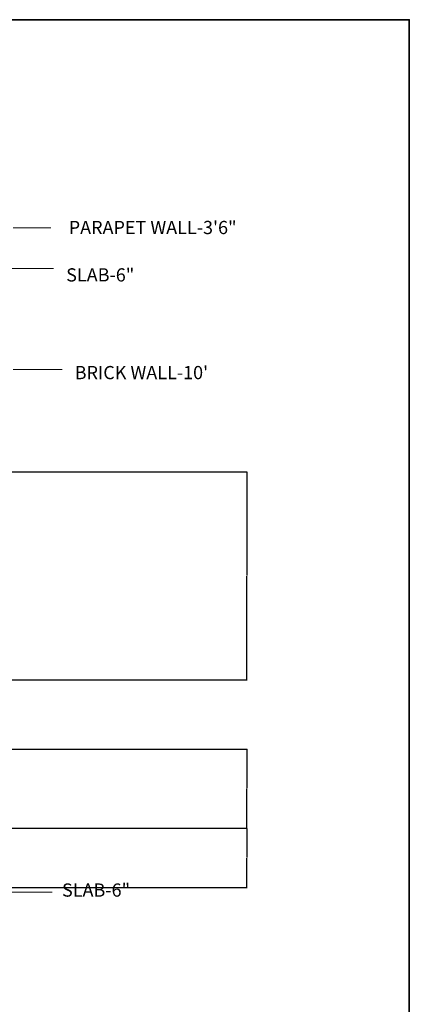
# Model space of a CAD drawing. Units: inches. Extents: x 1355 to 2746, y 1171 to 2751.
# Tile 24 of 24: x 2510 to 2746, y 2155 to 2751. Entities that reach past the tile are written whole.
import ezdxf

# ---------------------------------------------------------------- set-up
doc = ezdxf.new("R2010")
doc.units = ezdxf.units.IN
for name, color, linetype, lineweight in [('A-ANNO-DIMS', 2, 'Continuous', 18), ('A-ANNO-TEXT', 7, 'Continuous', 18), ('A-ANNO-TTLB', 7, 'Continuous', 35), ('A-WALL-PATT', 252, 'Continuous', 13)]:
    doc.layers.add(name, color=color, linetype=linetype, lineweight=lineweight)
doc.styles.get("Standard").update_dxf_attribs({"font": 'arial.ttf'})
doc.dimstyles.get("Standard").update_dxf_attribs({"dimtxt": 0.18, "dimasz": 0.18, "dimexe": 0.18, "dimexo": 0.0625, "dimgap": 0.09, "dimtad": 0, "dimtih": 1, "dimtoh": 1, "dimdec": 4, "dimzin": 0, "dimdsep": 46, "dimtxsty": 'Standard', "dimcen": 0.09, "dimadec": 0, "dimazin": 0, "dimtfac": 1, "dimtdec": 4, "dimtofl": 0, "dimtmove": 0, "dimatfit": 3, "dimfxl": 1, "dimtolj": 1, "dimtzin": 0, "dimarcsym": 0})

# ---------------------------------------------------------------- blocks, each defined once
blk = doc.blocks.new('*D116')
at = {"layer": 'A-ANNO-DIMS', "color": 0, "lineweight": -2, "transparency": 16777216}
for p, q in [((1976.77, 2477.4), (2648.07, 2477.4)), ((2647.89, 2477.22), (2647.89, 2414.58)), ((2647.89, 2351.58), (2647.89, 2414.22)), ((1976.77, 2351.4), (2648.07, 2351.4))]:
    blk.add_line(p, q, dxfattribs=at)
at = {"layer": 'A-ANNO-DIMS', "color": 0, "transparency": 16777216}
for points in [[(2647.86, 2477.22), (2647.92, 2477.22), (2647.89, 2477.4)], [(2647.86, 2351.58), (2647.92, 2351.58), (2647.89, 2351.4)]]:
    blk.add_solid(points, dxfattribs=at)
at = {"layer": 'Defpoints', "color": 0, "transparency": 16777216}
for p in [(1976.71, 2477.4), (2647.89, 2477.4), (1976.71, 2351.4)]:
    blk.add_point(p, dxfattribs=at)
at = {"layer": 'A-ANNO-DIMS', "color": 0, "transparency": 16777216, "insert": (2647.89, 2414.4), "char_height": 0.18, "attachment_point": 5}
blk.add_mtext('\\A1;126', dxfattribs=at)
blk = doc.blocks.new('*D123')
at = {"layer": 'A-ANNO-DIMS', "color": 0, "lineweight": -2, "transparency": 16777216}
for p, q in [((1880.77, 2261.4), (2648.07, 2261.4)), ((2647.89, 2261.22), (2647.89, 2243.58)), ((2647.89, 2225.58), (2647.89, 2243.22)), ((1940.77, 2225.4), (2648.07, 2225.4))]:
    blk.add_line(p, q, dxfattribs=at)
at = {"layer": 'A-ANNO-DIMS', "color": 0, "transparency": 16777216}
for points in [[(2647.86, 2261.22), (2647.92, 2261.22), (2647.89, 2261.4)], [(2647.86, 2225.58), (2647.92, 2225.58), (2647.89, 2225.4)]]:
    blk.add_solid(points, dxfattribs=at)
at = {"layer": 'Defpoints', "color": 0, "transparency": 16777216}
for p in [(1880.71, 2261.4), (2647.89, 2261.4), (1940.71, 2225.4)]:
    blk.add_point(p, dxfattribs=at)
at = {"layer": 'A-ANNO-DIMS', "color": 0, "transparency": 16777216, "insert": (2647.89, 2243.4), "char_height": 0.18, "attachment_point": 5}
blk.add_mtext('\\A1;36', dxfattribs=at)
blk = doc.blocks.new('*D125')
at = {"layer": 'A-ANNO-DIMS', "color": 0, "lineweight": -2, "transparency": 16777216}
for p, q in [((1880.77, 2309.4), (2648.07, 2309.4)), ((2647.89, 2309.22), (2647.89, 2285.58)), ((2647.89, 2261.58), (2647.89, 2285.22)), ((1880.77, 2261.4), (2648.07, 2261.4))]:
    blk.add_line(p, q, dxfattribs=at)
at = {"layer": 'A-ANNO-DIMS', "color": 0, "transparency": 16777216}
for points in [[(2647.86, 2309.22), (2647.92, 2309.22), (2647.89, 2309.4)], [(2647.86, 2261.58), (2647.92, 2261.58), (2647.89, 2261.4)]]:
    blk.add_solid(points, dxfattribs=at)
at = {"layer": 'Defpoints', "color": 0, "transparency": 16777216}
for p in [(1880.71, 2309.4), (2647.89, 2309.4), (1880.71, 2261.4)]:
    blk.add_point(p, dxfattribs=at)
at = {"layer": 'A-ANNO-DIMS', "color": 0, "transparency": 16777216, "insert": (2647.89, 2285.4), "char_height": 0.18, "attachment_point": 5}
blk.add_mtext('\\A1;48', dxfattribs=at)
blk = doc.blocks.new('*D128')
at = {"layer": 'A-ANNO-DIMS', "color": 0, "lineweight": -2, "transparency": 16777216}
for p, q in [((2506.45, 2477.4), (2648.07, 2477.4)), ((2647.89, 2477.22), (2647.89, 2414.58)), ((2647.89, 2351.58), (2647.89, 2414.22)), ((2506.45, 2351.4), (2648.07, 2351.4))]:
    blk.add_line(p, q, dxfattribs=at)
at = {"layer": 'A-ANNO-DIMS', "color": 0, "transparency": 16777216}
for points in [[(2647.86, 2477.22), (2647.92, 2477.22), (2647.89, 2477.4)], [(2647.86, 2351.58), (2647.92, 2351.58), (2647.89, 2351.4)]]:
    blk.add_solid(points, dxfattribs=at)
at = {"layer": 'Defpoints', "color": 0, "transparency": 16777216}
for p in [(2506.39, 2477.4), (2647.89, 2477.4), (2506.39, 2351.4)]:
    blk.add_point(p, dxfattribs=at)
at = {"layer": 'A-ANNO-DIMS', "color": 0, "transparency": 16777216, "insert": (2647.89, 2414.4), "char_height": 0.18, "attachment_point": 5}
blk.add_mtext('\\A1;126', dxfattribs=at)

msp = doc.modelspace()

# ---------------------------------------------------------------- hatches: boundary and pattern name
at = {"layer": 'A-WALL-PATT'}
h = msp.add_hatch(dxfattribs=at)
h.set_pattern_fill('ANSI32', color=256)
h.paths.add_polyline_path([(1660.2083, 2139.3018), (1614.5977, 2139.3018), (1614.5977, 2130.3018), (1655.7083, 2130.3018), (1655.7083, 1981.8018), (1660.2083, 1981.8018), (1660.2083, 2090.7225), (1692.5832, 2090.7225), (1692.5832, 2095.2225), (1660.2083, 2095.2225)])
h.paths.add_polyline_path([(1523.7083, 2130.3018), (1554.5977, 2130.3018), (1554.5977, 2134.8018), (1554.5977, 2139.3018), (1514.7083, 2139.3018), (1514.7083, 2071.8385), (1523.7083, 2071.8385)])
h.paths.add_polyline_path([(1940.7083, 2139.3018), (1883.7928, 2139.3018), (1883.7928, 2130.3018), (1931.7083, 2130.3018), (1931.7083, 2098.3333), (1940.7083, 2098.3333)])
h.paths.add_polyline_path([(1799.7083, 2130.3018), (1823.7928, 2130.3018), (1823.7928, 2134.8018), (1823.7928, 2139.3018), (1795.2083, 2139.3018), (1795.2083, 2130.3018), (1795.2083, 2095.2225), (1759.2134, 2095.2225), (1759.2134, 2090.7225), (1795.2083, 2090.7225), (1795.2083, 1981.8018), (1799.7083, 1981.8018), (1799.7083, 1986.3018)])
h.paths.add_polyline_path([(1940.7083, 2038.3333), (1931.7083, 2038.3333), (1931.7083, 1986.3018), (1832.7083, 1986.3018), (1832.7083, 1947.1338), (1837.2083, 1947.1338), (1837.2083, 1981.8018), (1931.7083, 1981.8018), (1931.7083, 1967.1939), (1940.7083, 1967.1939)])
h.paths.add_polyline_path([(1940.7083, 1943.1939), (1931.7083, 1943.1939), (1931.7083, 1921.8018), (1837.2083, 1921.8018), (1837.2083, 1926.0511), (1832.7083, 1926.0511), (1832.7083, 1917.3018), (1931.7083, 1917.3018), (1931.7083, 1908.3321), (1940.7083, 1908.3321)])
h.paths.add_polyline_path([(1940.7083, 1884.3321), (1931.7083, 1884.3321), (1931.7083, 1869.3018), (1899.4583, 1869.3018), (1899.4583, 1864.8018), (1931.7083, 1864.8018), (1931.7083, 1773.3018), (1786.5143, 1773.3018), (1786.5143, 1764.3018), (1844.7083, 1764.3018), (1844.7083, 1748.9343), (1853.7083, 1748.9343), (1853.7083, 1764.3018), (1931.7083, 1764.3018), (1931.7083, 1652.9424), (1940.7083, 1652.9424)])
h.paths.add_polyline_path([(1799.7083, 1864.8018), (1806.0522, 1864.8018), (1806.0522, 1867.0518), (1806.0522, 1869.3018), (1799.7083, 1869.3018), (1799.7083, 1917.3018), (1799.7083, 1921.8018), (1795.2083, 1921.8018), (1795.2083, 1773.3018), (1799.7083, 1773.3018)])
h.paths.add_polyline_path([(1872.8988, 1867.0518), (1872.8988, 1869.3018), (1867.2083, 1869.3018), (1867.2083, 1917.3018), (1862.7083, 1917.3018), (1862.7083, 1869.3018), (1836.9546, 1869.3018), (1836.9546, 1864.8018), (1862.7083, 1864.8018), (1872.8988, 1864.8018)])
h.paths.add_polyline_path([(1749.2197, 1773.3018), (1655.7083, 1773.3018), (1523.7083, 1773.3018), (1523.7083, 1828.4963), (1514.7083, 1828.4963), (1514.7083, 1753.9033), (1519.2083, 1753.9033), (1523.7083, 1753.9033), (1523.7083, 1764.3018), (1655.7083, 1764.3018), (1749.2197, 1764.3018), (1749.2197, 1768.8018)])
h.paths.add_polyline_path([(1660.2083, 1921.8018), (1655.7083, 1921.8018), (1655.7083, 1917.3018), (1655.7083, 1773.3018), (1660.2083, 1773.3018)])
h.paths.add_polyline_path([(1523.7083, 2011.8385), (1514.7083, 2011.8385), (1514.7083, 1973.114), (1519.2083, 1973.114), (1523.7083, 1973.114), (1523.7083, 1976.8227), (1523.7083, 1981.8018), (1618.2083, 1981.8018), (1618.2083, 1921.8018), (1553.707, 1921.8018), (1553.707, 1917.3018), (1622.7083, 1917.3018), (1622.7083, 1919.5518), (1622.7083, 1921.8018), (1622.7083, 1986.3018), (1523.7083, 1986.3018)])
h.paths.add_polyline_path([(1529.6686, 1919.5518), (1529.6686, 1921.8018), (1523.7083, 1921.8018), (1523.7083, 1949.114), (1514.7083, 1949.114), (1514.7083, 1888.4963), (1523.7083, 1888.4963), (1523.7083, 1917.3018), (1529.6686, 1917.3018)])
h.paths.add_polyline_path([(1538.9419, 1775.643), (1585.5504, 1775.643), (1585.5504, 1798.0318), (1538.9419, 1798.0318)], flags=25)
h.paths.add_polyline_path([(1696.7097, 1497.3356), (1769.5651, 1497.3356), (1769.5651, 1523.4559), (1696.7097, 1523.4559)], flags=9)
h.paths.add_polyline_path([(1629.1643, 1230.5133), (1877.0879, 1230.5133), (1877.0879, 1267.606), (1629.1643, 1267.606)], flags=9)
h.paths.add_polyline_path([(2533.4462, 2215.4033), (2579.9292, 2215.4033), (2579.9292, 2231.889), (2533.4462, 2231.889)], flags=9)
h.paths.add_polyline_path([(2540.822, 2515.6945), (2594.2245, 2515.6945), (2594.2245, 2545.5463), (2540.822, 2545.5463)], flags=9)
h.paths.add_polyline_path([(2535.9857, 2588.2819), (2582.4687, 2588.2819), (2582.4687, 2604.7675), (2535.9857, 2604.7675)], flags=9)
h.paths.add_polyline_path([(2537.1627, 2617.1172), (2649.1245, 2617.1172), (2649.1245, 2633.6029), (2537.1627, 2633.6029)], flags=9)
h.paths.add_polyline_path([(2218.0051, 2168.228), (2363.9573, 2168.228), (2363.9573, 2205.3208), (2218.0051, 2205.3208)], flags=9)
h.paths.add_polyline_path([(1650.2156, 2165.3631), (1800.3547, 2165.3631), (1800.3547, 2202.4559), (1650.2156, 2202.4559)], flags=9)
h.paths.add_polyline_path([(2553.9592, 1610.7663), (2588.4203, 1610.7663), (2588.4203, 1660.2233), (2553.9592, 1660.2233)], flags=9)
h.paths.add_polyline_path([(1549.0868, 1648.2033), (1595.6952, 1648.2033), (1595.6952, 1670.5921), (1549.0868, 1670.5921)], flags=9)
h.paths.add_polyline_path([(1546.9525, 1502.0931), (1583.3413, 1502.0931), (1583.3413, 1524.4819), (1546.9525, 1524.4819)], flags=9)
h.paths.add_polyline_path([(1540.7704, 1433.4431), (1587.3788, 1433.4431), (1587.3788, 1455.8319), (1540.7704, 1455.8319)], flags=9)
h.paths.add_polyline_path([(1683.6524, 1321.5269), (1760.6169, 1321.5269), (1760.6169, 1333.8911), (1683.6524, 1333.8911)], flags=9)
h.paths.add_polyline_path([(1832.0485, 1356.0874), (1873.0989, 1356.0874), (1873.0989, 1378.4762), (1832.0485, 1378.4762)], flags=9)
h.paths.add_polyline_path([(1877.9694, 1431.2138), (1926.3827, 1431.2138), (1926.3827, 1453.578), (1877.9694, 1453.578)], flags=9)
h.paths.add_polyline_path([(1847.3106, 1499.8371), (1883.6994, 1499.8371), (1883.6994, 1522.2259), (1847.3106, 1522.2259)], flags=9)
h.paths.add_polyline_path([(1813.7015, 1640.7287), (1860.3099, 1640.7287), (1860.3099, 1663.1175), (1813.7015, 1663.1175)], flags=9)
h.paths.add_polyline_path([(1876.2576, 1710.2471), (1912.9452, 1710.2471), (1912.9452, 1732.6359), (1876.2576, 1732.6359)], flags=25)
h.paths.add_polyline_path([(1695.9163, 1715.3064), (1736.9668, 1715.3064), (1736.9668, 1737.6952), (1695.9163, 1737.6952)], flags=9)
h.paths.add_polyline_path([(1881.8583, 1888.9094), (1930.2717, 1888.9094), (1930.2717, 1911.2737), (1881.8583, 1911.2737)], flags=9)
h.paths.add_polyline_path([(1823.9298, 1798.6431), (1864.9803, 1798.6431), (1864.9803, 1821.0319), (1823.9298, 1821.0319)], flags=25)
h.paths.add_polyline_path([(1845.6062, 1948.1408), (1881.995, 1948.1408), (1881.995, 1970.5296), (1845.6062, 1970.5296)], flags=25)
h.paths.add_polyline_path([(1849.027, 1991.5151), (1895.6355, 1991.5151), (1895.6355, 2013.9039), (1849.027, 2013.9039)], flags=25)
h.paths.add_polyline_path([(1684.9725, 2113.8416), (1764.2658, 2113.8416), (1764.2658, 2126.2058), (1684.9725, 2126.2058)], flags=9)
h.paths.add_polyline_path([(1688.6193, 1913.0676), (1776.2005, 1913.0676), (1776.2005, 1935.4564), (1688.6193, 1935.4564)], flags=9)
h.paths.add_polyline_path([(1571.4689, 1930.9816), (1607.8577, 1930.9816), (1607.8577, 1953.3704), (1571.4689, 1953.3704)], flags=25)
h.paths.add_polyline_path([(1535.3581, 1998.3125), (1581.9665, 1998.3125), (1581.9665, 2020.7014), (1535.3581, 2020.7014)], flags=9)
h = msp.add_hatch(dxfattribs=at)
h.set_pattern_fill('ANSI32', color=256)
h.paths.add_polyline_path([(1749.2197, 1686.3018), (1732.6892, 1686.3018), (1523.7083, 1686.3018), (1523.7083, 1705.9033), (1514.7083, 1705.9033), (1514.7083, 1647.8732), (1519.2083, 1647.8732), (1523.7083, 1647.8732), (1523.7083, 1677.3018), (1655.7083, 1677.3018), (1655.7083, 1528.8018), (1660.2083, 1528.8018), (1660.2083, 1677.3018), (1732.6892, 1677.3018), (1749.2197, 1677.3018)])
h.paths.add_polyline_path([(1931.7083, 1686.3018), (1853.7083, 1686.3018), (1853.7083, 1703.5696), (1844.7083, 1703.5696), (1844.7083, 1686.3018), (1788.0274, 1686.3018), (1788.0274, 1677.3018), (1795.2083, 1677.3018), (1795.2083, 1528.8018), (1799.7083, 1528.8018), (1799.7083, 1677.3018), (1844.7083, 1677.3018), (1931.7083, 1677.3018)])
h.paths.add_polyline_path([(1931.7083, 1533.3018), (1844.7083, 1533.3018), (1832.7083, 1533.3018), (1832.7083, 1531.0518), (1832.7083, 1528.8018), (1832.7083, 1495.7519), (1837.2083, 1495.7519), (1837.2083, 1528.8018), (1931.7083, 1528.8018)])
h.paths.add_polyline_path([(1940.7083, 1592.9424), (1931.7083, 1592.9424), (1931.7083, 1506.7845), (1940.7083, 1506.7845)])
h.paths.add_polyline_path([(1940.7083, 1482.7845), (1936.2083, 1482.7845), (1931.7083, 1482.7845), (1931.7083, 1320.3018), (1880.7083, 1320.3018), (1880.7083, 1311.3018), (1940.7083, 1311.3018)])
h.paths.add_polyline_path([(1931.7083, 1468.8018), (1844.7083, 1468.8018), (1837.2083, 1468.8018), (1837.2083, 1474.34), (1832.7083, 1474.34), (1832.7083, 1468.8018), (1832.7083, 1464.3018), (1844.7083, 1464.3018), (1931.7083, 1464.3018)])
h.paths.add_polyline_path([(1863.8571, 1464.3018), (1859.3571, 1464.3018), (1859.3571, 1404.1662), (1838.1542, 1404.1662), (1838.1542, 1399.8018), (1869.4185, 1399.8018), (1869.4185, 1402.0518), (1869.4185, 1404.3018), (1863.8571, 1404.3018)])
h.paths.add_polyline_path([(1799.7083, 1399.6662), (1805.4082, 1399.6662), (1805.4082, 1401.9162), (1805.4082, 1404.1662), (1799.7083, 1404.1662), (1799.7083, 1464.3018), (1799.7083, 1468.8018), (1795.2083, 1468.8018), (1795.2083, 1356.2098), (1761.2597, 1356.2098), (1761.2597, 1351.7098), (1795.2083, 1351.7098), (1795.2083, 1320.3018), (1795.2083, 1311.3018), (1844.7083, 1311.3018), (1844.7083, 1315.8018), (1844.7083, 1320.3018), (1799.7083, 1320.3018)])
h.paths.add_polyline_path([(1692.9218, 1356.2098), (1660.2083, 1356.2098), (1660.2083, 1430.786), (1657.9583, 1430.786), (1655.7083, 1430.786), (1655.7083, 1320.3018), (1611.934, 1320.3018), (1611.934, 1311.3018), (1660.2083, 1311.3018), (1660.2083, 1351.7098), (1692.9218, 1351.7098)])
h.paths.add_polyline_path([(1523.7083, 1372.653), (1514.7083, 1372.653), (1514.7083, 1311.3018), (1551.934, 1311.3018), (1551.934, 1315.8018), (1551.934, 1320.3018), (1523.7083, 1320.3018)])
h.paths.add_polyline_path([(1523.7083, 1490.9023), (1514.7083, 1490.9023), (1514.7083, 1432.653), (1519.2083, 1432.653), (1523.7083, 1432.653)])
h.paths.add_polyline_path([(1660.2083, 1468.8018), (1622.7083, 1468.8018), (1622.7083, 1473.1566), (1618.2083, 1473.1566), (1618.2083, 1468.8018), (1523.7083, 1468.8018), (1523.7083, 1464.3018), (1655.7083, 1464.3018), (1655.7083, 1460.5634), (1660.2083, 1460.5634)])
h.paths.add_polyline_path([(1523.7083, 1587.8732), (1514.7083, 1587.8732), (1514.7083, 1514.9023), (1519.2083, 1514.9023), (1523.7083, 1514.9023)])
h.paths.add_polyline_path([(1622.7083, 1533.3018), (1523.7083, 1533.3018), (1523.7083, 1528.8018), (1618.2083, 1528.8018), (1618.2083, 1494.4205), (1622.7083, 1494.4205), (1622.7083, 1528.8018)])
h.paths.add_polyline_path([(1696.7097, 1497.3356), (1769.5651, 1497.3356), (1769.5651, 1523.4559), (1696.7097, 1523.4559)], flags=9)
h.paths.add_polyline_path([(1629.1643, 1230.5133), (1877.0879, 1230.5133), (1877.0879, 1267.606), (1629.1643, 1267.606)], flags=9)
h.paths.add_polyline_path([(2533.4462, 2215.4033), (2579.9292, 2215.4033), (2579.9292, 2231.889), (2533.4462, 2231.889)], flags=9)
h.paths.add_polyline_path([(2540.822, 2515.6945), (2594.2245, 2515.6945), (2594.2245, 2545.5463), (2540.822, 2545.5463)], flags=9)
h.paths.add_polyline_path([(2535.9857, 2588.2819), (2582.4687, 2588.2819), (2582.4687, 2604.7675), (2535.9857, 2604.7675)], flags=9)
h.paths.add_polyline_path([(2537.1627, 2617.1172), (2649.1245, 2617.1172), (2649.1245, 2633.6029), (2537.1627, 2633.6029)], flags=9)
h.paths.add_polyline_path([(2218.0051, 2168.228), (2363.9573, 2168.228), (2363.9573, 2205.3208), (2218.0051, 2205.3208)], flags=9)
h.paths.add_polyline_path([(1650.2156, 2165.3631), (1800.3547, 2165.3631), (1800.3547, 2202.4559), (1650.2156, 2202.4559)], flags=9)
h.paths.add_polyline_path([(2553.9592, 1610.7663), (2588.4203, 1610.7663), (2588.4203, 1660.2233), (2553.9592, 1660.2233)], flags=9)
h.paths.add_polyline_path([(1549.0868, 1648.2033), (1595.6952, 1648.2033), (1595.6952, 1670.5921), (1549.0868, 1670.5921)], flags=25)
h.paths.add_polyline_path([(1546.9525, 1502.0931), (1583.3413, 1502.0931), (1583.3413, 1524.4819), (1546.9525, 1524.4819)], flags=25)
h.paths.add_polyline_path([(1540.7704, 1433.4431), (1587.3788, 1433.4431), (1587.3788, 1455.8319), (1540.7704, 1455.8319)], flags=9)
h.paths.add_polyline_path([(1683.6524, 1321.5269), (1760.6169, 1321.5269), (1760.6169, 1333.8911), (1683.6524, 1333.8911)], flags=9)
h.paths.add_polyline_path([(1832.0485, 1356.0874), (1873.0989, 1356.0874), (1873.0989, 1378.4762), (1832.0485, 1378.4762)], flags=9)
h.paths.add_polyline_path([(1877.9694, 1431.2138), (1926.3827, 1431.2138), (1926.3827, 1453.578), (1877.9694, 1453.578)], flags=9)
h.paths.add_polyline_path([(1847.3106, 1499.8371), (1883.6994, 1499.8371), (1883.6994, 1522.2259), (1847.3106, 1522.2259)], flags=25)
h.paths.add_polyline_path([(1813.7015, 1640.7287), (1860.3099, 1640.7287), (1860.3099, 1663.1175), (1813.7015, 1663.1175)], flags=25)
h.paths.add_polyline_path([(1876.2576, 1710.2471), (1912.9452, 1710.2471), (1912.9452, 1732.6359), (1876.2576, 1732.6359)], flags=9)
h.paths.add_polyline_path([(1695.9163, 1715.3064), (1736.9668, 1715.3064), (1736.9668, 1737.6952), (1695.9163, 1737.6952)], flags=9)
h.paths.add_polyline_path([(1881.8583, 1888.9094), (1930.2717, 1888.9094), (1930.2717, 1911.2737), (1881.8583, 1911.2737)], flags=9)
h.paths.add_polyline_path([(1823.9298, 1798.6431), (1864.9803, 1798.6431), (1864.9803, 1821.0319), (1823.9298, 1821.0319)], flags=9)
h.paths.add_polyline_path([(1845.6062, 1948.1408), (1881.995, 1948.1408), (1881.995, 1970.5296), (1845.6062, 1970.5296)], flags=9)
h.paths.add_polyline_path([(1849.027, 1991.5151), (1895.6355, 1991.5151), (1895.6355, 2013.9039), (1849.027, 2013.9039)], flags=9)
h.paths.add_polyline_path([(1684.9725, 2113.8416), (1764.2658, 2113.8416), (1764.2658, 2126.2058), (1684.9725, 2126.2058)], flags=9)
h.paths.add_polyline_path([(1688.6193, 1913.0676), (1776.2005, 1913.0676), (1776.2005, 1935.4564), (1688.6193, 1935.4564)], flags=9)
h.paths.add_polyline_path([(1538.9419, 1775.643), (1585.5504, 1775.643), (1585.5504, 1798.0318), (1538.9419, 1798.0318)], flags=9)
h.paths.add_polyline_path([(1571.4689, 1930.9816), (1607.8577, 1930.9816), (1607.8577, 1953.3704), (1571.4689, 1953.3704)], flags=9)
h.paths.add_polyline_path([(1535.3581, 1998.3125), (1581.9665, 1998.3125), (1581.9665, 2020.7014), (1535.3581, 2020.7014)], flags=9)

# ---------------------------------------------------------------- linework, layer by layer
at = {"layer": 'A-ANNO-TEXT'}
for p, q in [((2506.3909, 2625.3279), (2529.1047, 2625.3279)), ((2502.5164, 2600.7394), (2530.7325, 2600.7394)), ((2506.3909, 2539.5356), (2536.1371, 2539.5356)), ((2502.4601, 2222.5737), (2530.0611, 2222.5737))]:
    msp.add_line(p, q, dxfattribs=at)
at = {"layer": 'A-ANNO-TTLB'}
msp.add_lwpolyline([(1355.0901, 2751.4741), (2746.1804, 2751.4741), (2746.1804, 1182.883), (1355.0901, 1182.883)], close=True, dxfattribs=at)

# ---------------------------------------------------------------- texts
at = {"layer": 'A-ANNO-TEXT', "char_height": 8, "attachment_point": 1}
for s, width, insert in [('PARAPET WALL-3\'6"', 118.662994, (2540.0249, 2629.5183)), ('SLAB-6"', 54.566591, (2538.4878, 2600.7866)), ("BRICK WALL-10'", 82.237335, (2543.6406, 2541.5654)), ('SLAB-6"', 35.745225, (2535.9483, 2227.9081))]:
    msp.add_mtext_dynamic_manual_height_columns(s, width=width, gutter_width=12.5, heights=[0], dxfattribs=dict(at, insert=insert))

# ---------------------------------------------------------------- dimensions: what is measured, and where the dimension line sits
at = {"layer": 'A-ANNO-DIMS'}
for base, p1, p2, picture, middle in [((2647.886, 2477.3999), (1976.7083, 2351.3999), (1976.7083, 2477.3999), '*D116', (2647.886, 2414.3999)), ((2647.886, 2477.3999), (2506.3909, 2351.3999), (2506.3909, 2477.3999), '*D128', (2647.886, 2414.3999)), ((2647.886, 2309.3999), (1880.7083, 2261.3999), (1880.7083, 2309.3999), '*D125', (2647.886, 2285.3999)), ((2647.886, 2261.3999), (1940.7083, 2225.3999), (1880.7083, 2261.3999), '*D123', (2647.886, 2243.3999))]:
    dim = msp.add_linear_dim(base=base, p1=p1, p2=p2, angle=90, dimstyle='Standard', override={"dimdec": 0, "dimlfac": 1, "dimrnd": 0, "dimzin": 0, "dimdsep": 46, "dimlunit": 2}, dxfattribs=at)
    dim.commit()
    dim.dimension.update_dxf_attribs({"geometry": picture, "text_midpoint": middle})

doc.saveas('drawing.dxf')
